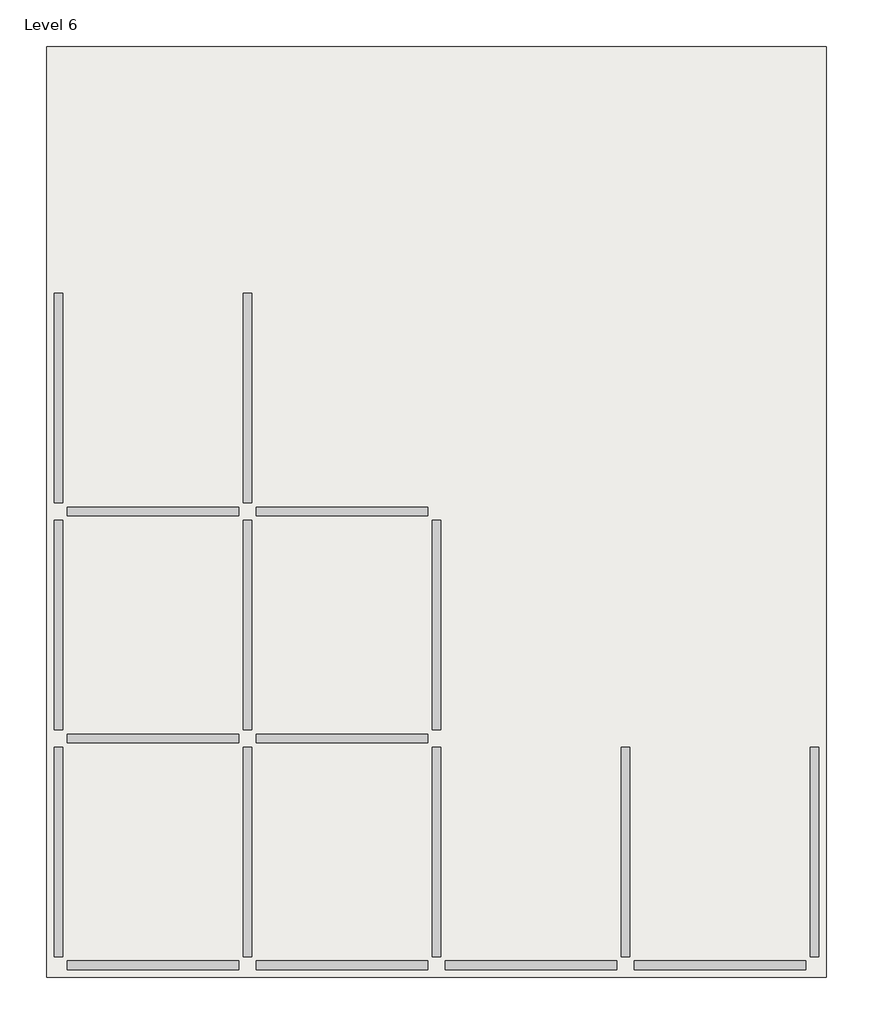
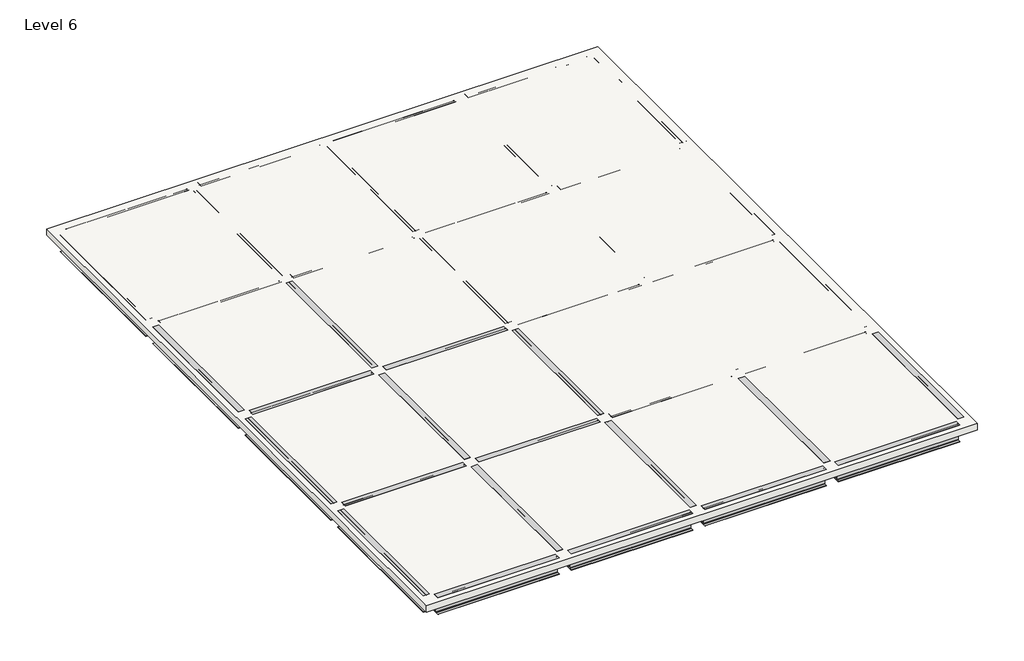
# One storey: 40 beams, 1 slab.
"""IFC4 building model written with IfcOpenShell, lengths in millimetres."""

from ifc_helpers import new_model, si_unit, frame, origin, place, context, project, spatial, polyline, outline, extrude, transform, mapped, element, save
from components import w_shapes_w16x26_71b85d0e, w_shapes_w16x26_5730d789

model = new_model("IFC4")

# Units and contexts
model_context = context("Model", 3, world=origin())
ifc_project = project(units=[si_unit("LENGTHUNIT", "METRE", prefix="MILLI")], contexts=[model_context])

# Site, building, storey
site = spatial("IfcSite", under=ifc_project)
building = spatial("IfcBuilding", under=site)
storey = spatial("IfcBuildingStorey", under=building, Name="Level 6", Elevation=15240.0)

# Beams
placement = place(None, origin())
w_shapes_w16x26_shape = w_shapes_w16x26_71b85d0e(model_context)
element("IfcBeam", 1, ObjectType="W Shapes : W16X26", at=placement, inside=storey, context=model_context, shape_type="MappedRepresentation", body=[
    mapped(w_shapes_w16x26_shape, transform((-5883.5186598, -2213.7239423, 15040.61), x_axis=(1.0, 0.0, 0.0), y_axis=(0.0, 1.0, 0.0), z_axis=(0.0, 0.0, 1.0))),
])
element("IfcBeam", 2, ObjectType="W Shapes : W16X26", at=placement, inside=storey, context=model_context, shape_type="MappedRepresentation", body=[
    mapped(w_shapes_w16x26_shape, transform((-2835.5186598, -2213.7239423, 15040.61), x_axis=(1.0, 0.0, 0.0), y_axis=(0.0, 1.0, 0.0), z_axis=(0.0, 0.0, 1.0))),
])
element("IfcBeam", 3, ObjectType="W Shapes : W16X26", at=placement, inside=storey, context=model_context, shape_type="MappedRepresentation", body=[
    mapped(w_shapes_w16x26_shape, transform((212.4813402, -2213.7239423, 15040.61), x_axis=(1.0, 0.0, 0.0), y_axis=(0.0, 1.0, 0.0), z_axis=(0.0, 0.0, 1.0))),
])
element("IfcBeam", 4, ObjectType="W Shapes : W16X26", at=placement, inside=storey, context=model_context, shape_type="MappedRepresentation", body=[
    mapped(w_shapes_w16x26_shape, transform((3260.4813402, -2213.7239423, 15040.61), x_axis=(1.0, 0.0, 0.0), y_axis=(0.0, 1.0, 0.0), z_axis=(0.0, 0.0, 1.0))),
])
element("IfcBeam", 5, ObjectType="W Shapes : W16X26", at=placement, inside=storey, context=model_context, shape_type="MappedRepresentation", body=[
    mapped(w_shapes_w16x26_shape, transform((-5883.5186598, 1443.8760577, 15040.61), x_axis=(1.0, 0.0, 0.0), y_axis=(0.0, 1.0, 0.0), z_axis=(0.0, 0.0, 1.0))),
])
element("IfcBeam", 6, ObjectType="W Shapes : W16X26", at=placement, inside=storey, context=model_context, shape_type="MappedRepresentation", body=[
    mapped(w_shapes_w16x26_shape, transform((-2835.5186598, 1443.8760577, 15040.61), x_axis=(1.0, 0.0, 0.0), y_axis=(0.0, 1.0, 0.0), z_axis=(0.0, 0.0, 1.0))),
])
element("IfcBeam", 7, ObjectType="W Shapes : W16X26", at=placement, inside=storey, context=model_context, shape_type="MappedRepresentation", body=[
    mapped(w_shapes_w16x26_shape, transform((212.4813402, 1443.8760577, 15040.61), x_axis=(1.0, 0.0, 0.0), y_axis=(0.0, 1.0, 0.0), z_axis=(0.0, 0.0, 1.0))),
])
element("IfcBeam", 8, ObjectType="W Shapes : W16X26", at=placement, inside=storey, context=model_context, shape_type="MappedRepresentation", body=[
    mapped(w_shapes_w16x26_shape, transform((3260.4813402, 1443.8760577, 15040.61), x_axis=(1.0, 0.0, 0.0), y_axis=(0.0, 1.0, 0.0), z_axis=(0.0, 0.0, 1.0))),
])
element("IfcBeam", 9, ObjectType="W Shapes : W16X26", at=placement, inside=storey, context=model_context, shape_type="MappedRepresentation", body=[
    mapped(w_shapes_w16x26_shape, transform((-5883.5186598, 5101.4760577, 15040.61), x_axis=(1.0, 0.0, 0.0), y_axis=(0.0, 1.0, 0.0), z_axis=(0.0, 0.0, 1.0))),
])
element("IfcBeam", 10, ObjectType="W Shapes : W16X26", at=placement, inside=storey, context=model_context, shape_type="MappedRepresentation", body=[
    mapped(w_shapes_w16x26_shape, transform((-2835.5186598, 5101.4760577, 15040.61), x_axis=(1.0, 0.0, 0.0), y_axis=(0.0, 1.0, 0.0), z_axis=(0.0, 0.0, 1.0))),
])
element("IfcBeam", 11, ObjectType="W Shapes : W16X26", at=placement, inside=storey, context=model_context, shape_type="MappedRepresentation", body=[
    mapped(w_shapes_w16x26_shape, transform((212.4813402, 5101.4760577, 15040.61), x_axis=(1.0, 0.0, 0.0), y_axis=(0.0, 1.0, 0.0), z_axis=(0.0, 0.0, 1.0))),
])
element("IfcBeam", 12, ObjectType="W Shapes : W16X26", at=placement, inside=storey, context=model_context, shape_type="MappedRepresentation", body=[
    mapped(w_shapes_w16x26_shape, transform((3260.4813402, 5101.4760577, 15040.61), x_axis=(1.0, 0.0, 0.0), y_axis=(0.0, 1.0, 0.0), z_axis=(0.0, 0.0, 1.0))),
])
element("IfcBeam", 13, ObjectType="W Shapes : W16X26", at=placement, inside=storey, context=model_context, shape_type="MappedRepresentation", body=[
    mapped(w_shapes_w16x26_shape, transform((-5883.5186598, 8759.0760577, 15040.61), x_axis=(1.0, 0.0, 0.0), y_axis=(0.0, 1.0, 0.0), z_axis=(0.0, 0.0, 1.0))),
])
element("IfcBeam", 14, ObjectType="W Shapes : W16X26", at=placement, inside=storey, context=model_context, shape_type="MappedRepresentation", body=[
    mapped(w_shapes_w16x26_shape, transform((-2835.5186598, 8759.0760577, 15040.61), x_axis=(1.0, 0.0, 0.0), y_axis=(0.0, 1.0, 0.0), z_axis=(0.0, 0.0, 1.0))),
])
element("IfcBeam", 15, ObjectType="W Shapes : W16X26", at=placement, inside=storey, context=model_context, shape_type="MappedRepresentation", body=[
    mapped(w_shapes_w16x26_shape, transform((212.4813402, 8759.0760577, 15040.61), x_axis=(1.0, 0.0, 0.0), y_axis=(0.0, 1.0, 0.0), z_axis=(0.0, 0.0, 1.0))),
])
element("IfcBeam", 16, ObjectType="W Shapes : W16X26", at=placement, inside=storey, context=model_context, shape_type="MappedRepresentation", body=[
    mapped(w_shapes_w16x26_shape, transform((3260.4813402, 8759.0760577, 15040.61), x_axis=(1.0, 0.0, 0.0), y_axis=(0.0, 1.0, 0.0), z_axis=(0.0, 0.0, 1.0))),
])
element("IfcBeam", 17, ObjectType="W Shapes : W16X26", at=placement, inside=storey, context=model_context, shape_type="MappedRepresentation", body=[
    mapped(w_shapes_w16x26_shape, transform((-5883.5186598, 12416.6760577, 15040.61), x_axis=(1.0, 0.0, 0.0), y_axis=(0.0, 1.0, 0.0), z_axis=(0.0, 0.0, 1.0))),
])
element("IfcBeam", 18, ObjectType="W Shapes : W16X26", at=placement, inside=storey, context=model_context, shape_type="MappedRepresentation", body=[
    mapped(w_shapes_w16x26_shape, transform((-2835.5186598, 12416.6760577, 15040.61), x_axis=(1.0, 0.0, 0.0), y_axis=(0.0, 1.0, 0.0), z_axis=(0.0, 0.0, 1.0))),
])
element("IfcBeam", 19, ObjectType="W Shapes : W16X26", at=placement, inside=storey, context=model_context, shape_type="MappedRepresentation", body=[
    mapped(w_shapes_w16x26_shape, transform((212.4813402, 12416.6760577, 15040.61), x_axis=(1.0, 0.0, 0.0), y_axis=(0.0, 1.0, 0.0), z_axis=(0.0, 0.0, 1.0))),
])
element("IfcBeam", 20, ObjectType="W Shapes : W16X26", at=placement, inside=storey, context=model_context, shape_type="MappedRepresentation", body=[
    mapped(w_shapes_w16x26_shape, transform((3260.4813402, 12416.6760577, 15040.61), x_axis=(1.0, 0.0, 0.0), y_axis=(0.0, 1.0, 0.0), z_axis=(0.0, 0.0, 1.0))),
])
w_shapes_w16x26_2_shape = w_shapes_w16x26_5730d789(model_context)
element("IfcBeam", 21, ObjectType="W Shapes : W16X26", at=placement, inside=storey, context=model_context, shape_type="MappedRepresentation", body=[
    mapped(w_shapes_w16x26_2_shape, transform((4784.4813402, 10587.8760577, 15040.61), x_axis=(0.0, -1.0, 0.0), y_axis=(1.0, 0.0, 0.0), z_axis=(0.0, 0.0, 1.0))),
])
element("IfcBeam", 22, ObjectType="W Shapes : W16X26", at=placement, inside=storey, context=model_context, shape_type="MappedRepresentation", body=[
    mapped(w_shapes_w16x26_2_shape, transform((4784.4813402, 6930.2760577, 15040.61), x_axis=(0.0, -1.0, 0.0), y_axis=(1.0, 0.0, 0.0), z_axis=(0.0, 0.0, 1.0))),
])
element("IfcBeam", 23, ObjectType="W Shapes : W16X26", at=placement, inside=storey, context=model_context, shape_type="MappedRepresentation", body=[
    mapped(w_shapes_w16x26_2_shape, transform((4784.4813402, 3272.6760577, 15040.61), x_axis=(0.0, -1.0, 0.0), y_axis=(1.0, 0.0, 0.0), z_axis=(0.0, 0.0, 1.0))),
])
element("IfcBeam", 24, ObjectType="W Shapes : W16X26", at=placement, inside=storey, context=model_context, shape_type="MappedRepresentation", body=[
    mapped(w_shapes_w16x26_2_shape, transform((4784.4813402, -384.9239423, 15040.61), x_axis=(0.0, -1.0, 0.0), y_axis=(1.0, 0.0, 0.0), z_axis=(0.0, 0.0, 1.0))),
])
element("IfcBeam", 25, ObjectType="W Shapes : W16X26", at=placement, inside=storey, context=model_context, shape_type="MappedRepresentation", body=[
    mapped(w_shapes_w16x26_2_shape, transform((1736.4813402, 10587.8760577, 15040.61), x_axis=(0.0, -1.0, 0.0), y_axis=(1.0, 0.0, 0.0), z_axis=(0.0, 0.0, 1.0))),
])
element("IfcBeam", 26, ObjectType="W Shapes : W16X26", at=placement, inside=storey, context=model_context, shape_type="MappedRepresentation", body=[
    mapped(w_shapes_w16x26_2_shape, transform((1736.4813402, 6930.2760577, 15040.61), x_axis=(0.0, -1.0, 0.0), y_axis=(1.0, 0.0, 0.0), z_axis=(0.0, 0.0, 1.0))),
])
element("IfcBeam", 27, ObjectType="W Shapes : W16X26", at=placement, inside=storey, context=model_context, shape_type="MappedRepresentation", body=[
    mapped(w_shapes_w16x26_2_shape, transform((1736.4813402, 3272.6760577, 15040.61), x_axis=(0.0, -1.0, 0.0), y_axis=(1.0, 0.0, 0.0), z_axis=(0.0, 0.0, 1.0))),
])
element("IfcBeam", 28, ObjectType="W Shapes : W16X26", at=placement, inside=storey, context=model_context, shape_type="MappedRepresentation", body=[
    mapped(w_shapes_w16x26_2_shape, transform((1736.4813402, -384.9239423, 15040.61), x_axis=(0.0, -1.0, 0.0), y_axis=(1.0, 0.0, 0.0), z_axis=(0.0, 0.0, 1.0))),
])
element("IfcBeam", 29, ObjectType="W Shapes : W16X26", at=placement, inside=storey, context=model_context, shape_type="MappedRepresentation", body=[
    mapped(w_shapes_w16x26_2_shape, transform((-1311.5186598, 10587.8760577, 15040.61), x_axis=(0.0, -1.0, 0.0), y_axis=(1.0, 0.0, 0.0), z_axis=(0.0, 0.0, 1.0))),
])
element("IfcBeam", 30, ObjectType="W Shapes : W16X26", at=placement, inside=storey, context=model_context, shape_type="MappedRepresentation", body=[
    mapped(w_shapes_w16x26_2_shape, transform((-1311.5186598, 6930.2760577, 15040.61), x_axis=(0.0, -1.0, 0.0), y_axis=(1.0, 0.0, 0.0), z_axis=(0.0, 0.0, 1.0))),
])
element("IfcBeam", 31, ObjectType="W Shapes : W16X26", at=placement, inside=storey, context=model_context, shape_type="MappedRepresentation", body=[
    mapped(w_shapes_w16x26_2_shape, transform((-1311.5186598, 3272.6760577, 15040.61), x_axis=(0.0, -1.0, 0.0), y_axis=(1.0, 0.0, 0.0), z_axis=(0.0, 0.0, 1.0))),
])
element("IfcBeam", 32, ObjectType="W Shapes : W16X26", at=placement, inside=storey, context=model_context, shape_type="MappedRepresentation", body=[
    mapped(w_shapes_w16x26_2_shape, transform((-1311.5186598, -384.9239423, 15040.61), x_axis=(0.0, -1.0, 0.0), y_axis=(1.0, 0.0, 0.0), z_axis=(0.0, 0.0, 1.0))),
])
element("IfcBeam", 33, ObjectType="W Shapes : W16X26", at=placement, inside=storey, context=model_context, shape_type="MappedRepresentation", body=[
    mapped(w_shapes_w16x26_2_shape, transform((-4359.5186598, 10587.8760577, 15040.61), x_axis=(0.0, -1.0, 0.0), y_axis=(1.0, 0.0, 0.0), z_axis=(0.0, 0.0, 1.0))),
])
element("IfcBeam", 34, ObjectType="W Shapes : W16X26", at=placement, inside=storey, context=model_context, shape_type="MappedRepresentation", body=[
    mapped(w_shapes_w16x26_2_shape, transform((-4359.5186598, 6930.2760577, 15040.61), x_axis=(0.0, -1.0, 0.0), y_axis=(1.0, 0.0, 0.0), z_axis=(0.0, 0.0, 1.0))),
])
element("IfcBeam", 35, ObjectType="W Shapes : W16X26", at=placement, inside=storey, context=model_context, shape_type="MappedRepresentation", body=[
    mapped(w_shapes_w16x26_2_shape, transform((-4359.5186598, 3272.6760577, 15040.61), x_axis=(0.0, -1.0, 0.0), y_axis=(1.0, 0.0, 0.0), z_axis=(0.0, 0.0, 1.0))),
])
element("IfcBeam", 36, ObjectType="W Shapes : W16X26", at=placement, inside=storey, context=model_context, shape_type="MappedRepresentation", body=[
    mapped(w_shapes_w16x26_2_shape, transform((-4359.5186598, -384.9239423, 15040.61), x_axis=(0.0, -1.0, 0.0), y_axis=(1.0, 0.0, 0.0), z_axis=(0.0, 0.0, 1.0))),
])
element("IfcBeam", 37, ObjectType="W Shapes : W16X26", at=placement, inside=storey, context=model_context, shape_type="MappedRepresentation", body=[
    mapped(w_shapes_w16x26_2_shape, transform((-7407.5186598, 10587.8760577, 15040.61), x_axis=(0.0, -1.0, 0.0), y_axis=(1.0, 0.0, 0.0), z_axis=(0.0, 0.0, 1.0))),
])
element("IfcBeam", 38, ObjectType="W Shapes : W16X26", at=placement, inside=storey, context=model_context, shape_type="MappedRepresentation", body=[
    mapped(w_shapes_w16x26_2_shape, transform((-7407.5186598, 6930.2760577, 15040.61), x_axis=(0.0, -1.0, 0.0), y_axis=(1.0, 0.0, 0.0), z_axis=(0.0, 0.0, 1.0))),
])
element("IfcBeam", 39, ObjectType="W Shapes : W16X26", at=placement, inside=storey, context=model_context, shape_type="MappedRepresentation", body=[
    mapped(w_shapes_w16x26_2_shape, transform((-7407.5186598, 3272.6760577, 15040.61), x_axis=(0.0, -1.0, 0.0), y_axis=(1.0, 0.0, 0.0), z_axis=(0.0, 0.0, 1.0))),
])
element("IfcBeam", 40, ObjectType="W Shapes : W16X26", at=placement, inside=storey, context=model_context, shape_type="MappedRepresentation", body=[
    mapped(w_shapes_w16x26_2_shape, transform((-7407.5186598, -384.9239423, 15040.61), x_axis=(0.0, -1.0, 0.0), y_axis=(1.0, 0.0, 0.0), z_axis=(0.0, 0.0, 1.0))),
])

# Slab
element("IfcSlab", 41, ObjectType="6\" Foundation Slab", at=placement, inside=storey, context=model_context, shape_type="SweptSolid", body=[
    extrude(outline(polyline([(4974.3230176, 12600.4819642), (4974.3230176, -2410.9180358), (-7598.6769824, -2410.9180358), (-7598.6769824, 12600.4819642), (4974.3230176, 12600.4819642)])), frame((0.0, 0.0, 15087.6), z_axis=(0.0, 0.0, 1.0), x_axis=(1.0, 0.0, 0.0)), (0.0, 0.0, 1.0), 152.4),
])

save(model, "model.ifc")

# Revit data of these elements
# Type "W Shapes : W16X26"
#   Section Name Key = "W16x26"
#   Assembly Code = "B10"
#   Width = 5.500"
#   Web Thickness = 0.250"
#   Web Fillet = 0.402"
#   Warping Constant = 565.00 in⁶
#   Torsional Moment of Inertia = 0.262 in⁴
#   Section Area = 7.68 in²
#   Plastic Modulus weak axis = 5.48 in³
#   Plastic Modulus strong axis = 44.20 in³
#   Perimeter = 52.20 ft²/ft
#   Nominal Weight = 26.00 lbf/ft
#   Moment of Inertia weak axis = 9.59 in⁴
#   Moment of Inertia strong axis = 301.00 in⁴
#   Height = 15.700"
#   Flange Thickness = 0.345"
#   Elastic Modulus weak axis = 3.49 in³
#   Elastic Modulus strong axis = 38.40 in³
#   Centroid Vertical = 7.850"
#   Centroid Horizontal = 2.750"
#   Bolt Spacing = 0' - 3 1/2"
#   Length [instance default] = 5' - 0"
#   Structural Material [instance default] = Steel ASTM A992
#   Principal Axes Angle = 0
# Type "6\" Foundation Slab"
#   Layers, outside or top first: 0' - 6" "Concrete, Cast-in-Place gray" (function 1)
# Elements 1, 2, 3, 4, 5, 6, 7, 8, 9, 10, 11, 12, 13, 14, 15, 16, 17, 18, 19, 20, 21, 22, 23, 24, 25, 26, 27, 28, 29, 30, 31, 32, 33, 34, 35, 36, 37, 38, 39, 40 (IfcBeam, "W Shapes : W16X26")
#   Comments = ""
#   Structural Material = Steel ASTM A992
#   Phase Created = New Construction
#   Materials on its faces: "Steel ASTM A992"
# Element 41 (IfcSlab, "6\" Foundation Slab")
#   Height Offset From Level = 0' - 0"
#   built-in parameter 1001954 = 1
#   Phase Created = New Construction
#   Materials on its faces: "Concrete, Cast-in-Place gray"
# Materials
#   "Steel ASTM A992": class "Metal", colour RGB 199 199 199, transparency 0, Description = "Structural steel 50ksi", Cost = 0
#   "Concrete, Cast-in-Place gray": class "Concrete", colour RGB 192 192 192, transparency 0, Description = "Cast-in-place concrete", Cost = 0
